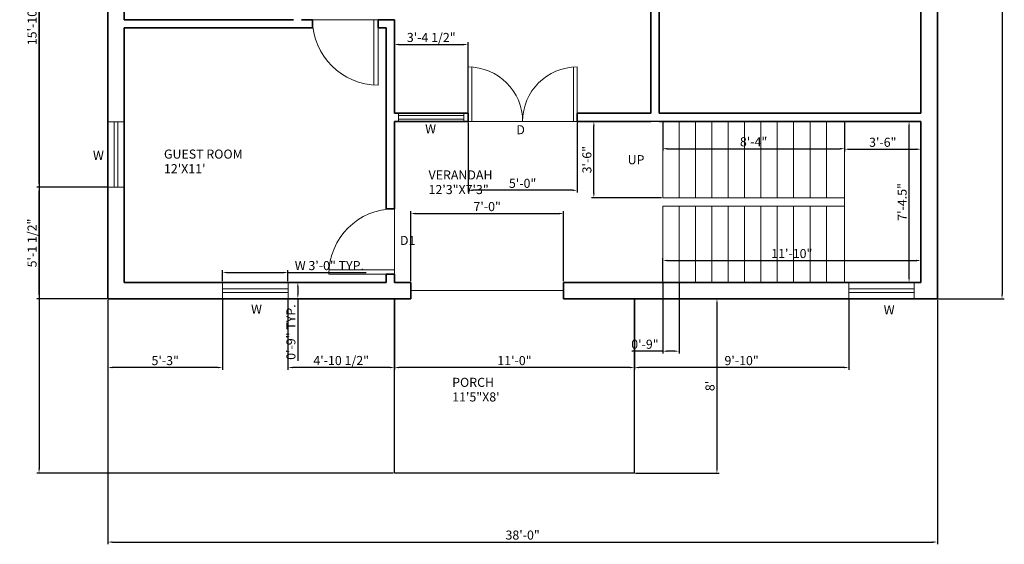
# Model space of a CAD drawing. Units: inches. Extents: x 2488 to 3029, y 1951 to 2721.
# Tile 1 of 2: x 2488 to 3029, y 1951 to 2239. Entities that reach past the tile are written whole.
import ezdxf

# ---------------------------------------------------------------- set-up
doc = ezdxf.new("R2010")
doc.units = ezdxf.units.IN
doc.header["$LTSCALE"] = 0.4
for name, color, linetype, lineweight in [('A-ANNO-DIMS', 52, 'Continuous', 18), ('A-ANNO-SYMB', 52, 'Continuous', 18), ('A-ANNO-TEXT', 52, 'Continuous', 18), ('A-AREA-IDEN', 52, 'Continuous', 18), ('A-FLOR-OTLN', 5, 'Continuous', 25), ('A-FLOR-STRS', 5, 'Continuous', 18), ('A-FLOR-THRS', 4, 'ZIGZAG', 18), ('A-GLAZ-JAMB', 8, 'ZIGZAG', 18), ('doors', 4, 'Continuous', 18), ('wall', 5, 'Continuous', 35), ('windows', 8, 'Continuous', 18)]:
    doc.layers.add(name, color=color, linetype=linetype, lineweight=lineweight)
doc.styles.get("Standard").update_dxf_attribs({"font": 'arial.ttf', "height": 5})
doc.linetypes.add('ZIGZAG', pattern='A,0.00254,-5.08,[131,ltypeshp.shx,S=5.08,R=0,X=-5.08,Y=0],-10.16,[131,ltypeshp.shx,S=5.08,R=180,X=5.08,Y=0],-5.08', length=20.32254)
doc.dimstyles.new('ISO-25', dxfattribs={"dimtxt": 5, "dimasz": 2.5, "dimexe": 1.25, "dimexo": 0.625, "dimtad": 1, "dimlunit": 3, "dimtxsty": 'Standard', "dimcen": 2.5, "dimadec": 0, "dimazin": 0, "dimtfac": 1, "dimtmove": 0, "dimatfit": 3, "dimfxl": 1, "dimarcsym": 0})

# ---------------------------------------------------------------- blocks, each defined once
blk = doc.blocks.new('*D1')
at = {"layer": 'A-ANNO-DIMS', "color": 0, "lineweight": -2, "transparency": 16777216}
for p, q in [((2841.37, 2182.57), (2841.37, 2166.96)), ((2941.37, 2182.57), (2941.37, 2166.96)), ((2843.87, 2168.21), (2938.87, 2168.21))]:
    blk.add_line(p, q, dxfattribs=at)
at = {"layer": 'A-ANNO-DIMS', "color": 0, "lineweight": 100, "transparency": 16777216}
for points in [[(2843.87, 2168.62), (2843.87, 2167.79), (2841.37, 2168.21)], [(2938.87, 2168.62), (2938.87, 2167.79), (2941.37, 2168.21)]]:
    blk.add_solid(points, dxfattribs=at)
at = {"layer": 'Defpoints', "color": 0, "lineweight": 100, "transparency": 16777216}
for p in [(2841.37, 2183.19), (2941.37, 2183.19), (2941.37, 2168.21)]:
    blk.add_point(p, dxfattribs=at)
at = {"layer": 'A-ANNO-DIMS', "color": 0, "transparency": 16777216, "insert": (2891.37, 2171.38), "char_height": 5, "attachment_point": 5}
blk.add_mtext('8\'-4"', dxfattribs=at)
blk = doc.blocks.new('*D2')
at = {"layer": 'A-ANNO-DIMS', "color": 0, "lineweight": -2, "transparency": 16777216}
for p, q in [((2941.37, 2182.57), (2941.37, 2166.68)), ((2983.37, 2182.57), (2983.37, 2166.68)), ((2943.87, 2167.93), (2980.87, 2167.93))]:
    blk.add_line(p, q, dxfattribs=at)
at = {"layer": 'A-ANNO-DIMS', "color": 0, "lineweight": 100, "transparency": 16777216}
for points in [[(2943.87, 2168.34), (2943.87, 2167.51), (2941.37, 2167.93)], [(2980.87, 2168.34), (2980.87, 2167.51), (2983.37, 2167.93)]]:
    blk.add_solid(points, dxfattribs=at)
at = {"layer": 'Defpoints', "color": 0, "lineweight": 100, "transparency": 16777216}
for p in [(2941.37, 2183.19), (2983.37, 2183.19), (2983.37, 2167.93)]:
    blk.add_point(p, dxfattribs=at)
at = {"layer": 'A-ANNO-DIMS', "color": 0, "transparency": 16777216, "insert": (2962.37, 2171.11), "char_height": 5, "attachment_point": 5}
blk.add_mtext('3\'-6"', dxfattribs=at)
blk = doc.blocks.new('*D3')
at = {"layer": 'A-ANNO-DIMS', "color": 0, "lineweight": -2, "transparency": 16777216}
for p, q in [((2982.75, 2183.19), (2975.57, 2183.19)), ((2976.82, 2097.19), (2976.82, 2180.69)), ((2982.75, 2094.69), (2975.57, 2094.69))]:
    blk.add_line(p, q, dxfattribs=at)
at = {"layer": 'A-ANNO-DIMS', "color": 0, "lineweight": 100, "transparency": 16777216}
for points in [[(2976.41, 2180.69), (2977.24, 2180.69), (2976.82, 2183.19)], [(2976.41, 2097.19), (2977.24, 2097.19), (2976.82, 2094.69)]]:
    blk.add_solid(points, dxfattribs=at)
at = {"layer": 'Defpoints', "color": 0, "lineweight": 100, "transparency": 16777216}
for p in [(2976.82, 2183.19), (2983.37, 2183.19), (2983.37, 2094.69)]:
    blk.add_point(p, dxfattribs=at)
at = {"layer": 'A-ANNO-DIMS', "color": 0, "transparency": 16777216, "insert": (2973.66, 2138.94), "char_height": 5, "attachment_point": 5, "rotation": 90}
blk.add_mtext('7\'-4.5"', dxfattribs=at)
blk = doc.blocks.new('*D4')
at = {"layer": 'A-ANNO-DIMS', "color": 0, "lineweight": -2, "transparency": 16777216}
for p, q in [((2841.37, 2095.32), (2841.37, 2107.97)), ((2843.87, 2106.72), (2980.87, 2106.72)), ((2983.37, 2095.32), (2983.37, 2107.97))]:
    blk.add_line(p, q, dxfattribs=at)
at = {"layer": 'A-ANNO-DIMS', "color": 0, "lineweight": 100, "transparency": 16777216}
for points in [[(2843.87, 2107.14), (2843.87, 2106.31), (2841.37, 2106.72)], [(2980.87, 2107.14), (2980.87, 2106.31), (2983.37, 2106.72)]]:
    blk.add_solid(points, dxfattribs=at)
at = {"layer": 'Defpoints', "color": 0, "lineweight": 100, "transparency": 16777216}
for p in [(2983.37, 2106.72), (2841.37, 2094.69), (2983.37, 2094.69)]:
    blk.add_point(p, dxfattribs=at)
at = {"layer": 'A-ANNO-DIMS', "color": 0, "transparency": 16777216, "insert": (2912.37, 2109.9), "char_height": 5, "attachment_point": 5}
blk.add_mtext('11\'-10"', dxfattribs=at)
blk = doc.blocks.new('*D5')
at = {"layer": 'A-ANNO-DIMS', "color": 0, "lineweight": -2, "transparency": 16777216}
for p, q in [((2826.5, 2085.69), (2872.45, 2085.69)), ((2871.2, 2083.19), (2871.2, 1992.19)), ((2826.5, 1989.69), (2872.45, 1989.69))]:
    blk.add_line(p, q, dxfattribs=at)
at = {"layer": 'A-ANNO-DIMS', "color": 0, "lineweight": 100, "transparency": 16777216}
for points in [[(2870.78, 2083.19), (2871.62, 2083.19), (2871.2, 2085.69)], [(2870.78, 1992.19), (2871.62, 1992.19), (2871.2, 1989.69)]]:
    blk.add_solid(points, dxfattribs=at)
at = {"layer": 'Defpoints', "color": 0, "lineweight": 100, "transparency": 16777216}
for p in [(2825.87, 2085.69), (2825.87, 1989.69), (2871.2, 1989.69)]:
    blk.add_point(p, dxfattribs=at)
at = {"layer": 'A-ANNO-DIMS', "color": 0, "transparency": 16777216, "insert": (2868.02, 2037.69), "char_height": 5, "attachment_point": 5, "rotation": 90}
blk.add_mtext("8'", dxfattribs=at)
blk = doc.blocks.new('*D6')
at = {"layer": 'A-ANNO-DIMS', "color": 0, "lineweight": -2, "transparency": 16777216}
for p, q in [((2993, 2625.69), (3029.19, 2625.69)), ((3027.94, 2623.19), (3027.94, 2088.19)), ((2993, 2085.69), (3029.19, 2085.69))]:
    blk.add_line(p, q, dxfattribs=at)
at = {"layer": 'A-ANNO-DIMS', "color": 0, "lineweight": 100, "transparency": 16777216}
for points in [[(3027.52, 2623.19), (3028.36, 2623.19), (3027.94, 2625.69)], [(3027.52, 2088.19), (3028.36, 2088.19), (3027.94, 2085.69)]]:
    blk.add_solid(points, dxfattribs=at)
at = {"layer": 'Defpoints', "color": 0, "lineweight": 100, "transparency": 16777216}
for p in [(2992.37, 2625.69), (2992.37, 2085.69), (3027.94, 2085.69)]:
    blk.add_point(p, dxfattribs=at)
at = {"layer": 'A-ANNO-DIMS', "color": 0, "transparency": 16777216, "insert": (3024.77, 2355.69), "char_height": 5, "attachment_point": 5, "rotation": 90}
blk.add_mtext("45'", dxfattribs=at)
blk = doc.blocks.new('WIN-36IN-9IN-WALL')
for p, q in [((0, 36), (0, 0)), ((9, 36), (0, 36)), ((3.5, 36), (3.5, 0)), ((5.5, 36), (5.5, 0)), ((9, 0), (9, 36)), ((0, 0), (9, 0))]:
    blk.add_line(p, q)
blk = doc.blocks.new('DOOR-SWING-30IN')
for p, q in [((28, 29.93), (28, 0)), ((30, 30), (30, 0)), ((30, 0), (0, 0))]:
    blk.add_line(p, q)
blk.add_arc((30, 0), 30, 90, 180)
blk = doc.blocks.new('DOOR-SWING-36IN')
for p, q in [((33.6, 35.92), (33.6, 0)), ((36, 36), (36, 0)), ((36, 0), (0, 0))]:
    blk.add_line(p, q)
blk.add_arc((36, 0), 36, 90, 180)
blk = doc.blocks.new('*D11')
at = {"layer": 'A-ANNO-DIMS', "color": 0, "lineweight": -2, "transparency": 16777216}
for p, q in [((2599.37, 2095.32), (2599.37, 2101.34)), ((2635.37, 2095.32), (2635.37, 2101.34)), ((2601.87, 2100.09), (2632.87, 2100.09)), ((2635.37, 2100.09), (2678.34, 2100.09))]:
    blk.add_line(p, q, dxfattribs=at)
at = {"layer": 'A-ANNO-DIMS', "color": 0, "lineweight": 100, "transparency": 16777216}
for points in [[(2601.87, 2100.51), (2601.87, 2099.68), (2599.37, 2100.09)], [(2632.87, 2100.51), (2632.87, 2099.68), (2635.37, 2100.09)]]:
    blk.add_solid(points, dxfattribs=at)
at = {"layer": 'Defpoints', "color": 0, "lineweight": 100, "transparency": 16777216}
for p in [(2635.37, 2100.09), (2599.37, 2094.69), (2635.37, 2094.69)]:
    blk.add_point(p, dxfattribs=at)
at = {"layer": 'A-ANNO-DIMS', "color": 0, "transparency": 16777216, "insert": (2658.11, 2103.27), "char_height": 5, "attachment_point": 5}
blk.add_mtext('W 3\'-0" TYP.', dxfattribs=at)
blk = doc.blocks.new('*D12')
at = {"layer": 'A-ANNO-DIMS', "color": 0, "lineweight": -2, "transparency": 16777216}
for p, q in [((2636, 2094.69), (2642.02, 2094.69)), ((2640.77, 2092.19), (2640.77, 2088.19)), ((2636, 2085.69), (2642.02, 2085.69)), ((2640.77, 2085.69), (2640.77, 2051.47))]:
    blk.add_line(p, q, dxfattribs=at)
at = {"layer": 'A-ANNO-DIMS', "color": 0, "lineweight": 100, "transparency": 16777216}
for points in [[(2640.36, 2092.19), (2641.19, 2092.19), (2640.77, 2094.69)], [(2640.36, 2088.19), (2641.19, 2088.19), (2640.77, 2085.69)]]:
    blk.add_solid(points, dxfattribs=at)
at = {"layer": 'Defpoints', "color": 0, "lineweight": 100, "transparency": 16777216}
for p in [(2635.37, 2094.69), (2635.37, 2085.69), (2640.77, 2085.69)]:
    blk.add_point(p, dxfattribs=at)
at = {"layer": 'A-ANNO-DIMS', "color": 0, "transparency": 16777216, "insert": (2637.6, 2067.33), "char_height": 5, "attachment_point": 5, "rotation": 90}
blk.add_mtext('0\'-9" TYP.', dxfattribs=at)
blk = doc.blocks.new('*D20')
at = {"layer": 'A-ANNO-DIMS', "color": 0, "lineweight": -2, "transparency": 16777216}
for p, q in [((2535.75, 2147.03), (2497.27, 2147.03)), ((2498.52, 2088.19), (2498.52, 2144.53)), ((2535.75, 2085.69), (2497.27, 2085.69))]:
    blk.add_line(p, q, dxfattribs=at)
at = {"layer": 'A-ANNO-DIMS', "color": 0, "lineweight": 100, "transparency": 16777216}
for points in [[(2498.11, 2144.53), (2498.94, 2144.53), (2498.52, 2147.03)], [(2498.11, 2088.19), (2498.94, 2088.19), (2498.52, 2085.69)]]:
    blk.add_solid(points, dxfattribs=at)
at = {"layer": 'Defpoints', "color": 0, "lineweight": 100, "transparency": 16777216}
for p in [(2498.52, 2147.03), (2536.37, 2147.03), (2536.37, 2085.69)]:
    blk.add_point(p, dxfattribs=at)
at = {"layer": 'A-ANNO-DIMS', "color": 0, "transparency": 16777216, "insert": (2495.31, 2116.36), "char_height": 5, "attachment_point": 5, "rotation": 90}
blk.add_mtext('5\'-1 1/2"', dxfattribs=at)
blk = doc.blocks.new('*D21')
at = {"layer": 'A-ANNO-DIMS', "color": 0, "lineweight": -2, "transparency": 16777216}
for p, q in [((2535.75, 2337.69), (2497.27, 2337.69)), ((2498.52, 2149.53), (2498.52, 2335.19)), ((2535.75, 2147.03), (2497.27, 2147.03))]:
    blk.add_line(p, q, dxfattribs=at)
at = {"layer": 'A-ANNO-DIMS', "color": 0, "lineweight": 100, "transparency": 16777216}
for points in [[(2498.11, 2335.19), (2498.94, 2335.19), (2498.52, 2337.69)], [(2498.11, 2149.53), (2498.94, 2149.53), (2498.52, 2147.03)]]:
    blk.add_solid(points, dxfattribs=at)
at = {"layer": 'Defpoints', "color": 0, "lineweight": 100, "transparency": 16777216}
for p in [(2498.52, 2337.69), (2536.37, 2337.69), (2536.37, 2147.03)]:
    blk.add_point(p, dxfattribs=at)
at = {"layer": 'A-ANNO-DIMS', "color": 0, "transparency": 16777216, "insert": (2495.31, 2242.36), "char_height": 5, "attachment_point": 5, "rotation": 90}
blk.add_mtext('15\'-10 1/2"', dxfattribs=at)
blk = doc.blocks.new('*D26')
at = {"layer": 'A-ANNO-DIMS', "color": 0, "lineweight": -2, "transparency": 16777216}
for p, q in [((2536.37, 2085.07), (2536.37, 2046.59)), ((2599.37, 2085.07), (2599.37, 2046.59)), ((2596.87, 2047.84), (2538.87, 2047.84))]:
    blk.add_line(p, q, dxfattribs=at)
at = {"layer": 'A-ANNO-DIMS', "color": 0, "lineweight": 100, "transparency": 16777216}
for points in [[(2538.87, 2048.26), (2538.87, 2047.43), (2536.37, 2047.84)], [(2596.87, 2048.26), (2596.87, 2047.43), (2599.37, 2047.84)]]:
    blk.add_solid(points, dxfattribs=at)
at = {"layer": 'Defpoints', "color": 0, "lineweight": 100, "transparency": 16777216}
for p in [(2536.37, 2085.69), (2599.37, 2085.69), (2536.37, 2047.84)]:
    blk.add_point(p, dxfattribs=at)
at = {"layer": 'A-ANNO-DIMS', "color": 0, "transparency": 16777216, "insert": (2567.87, 2051.02), "char_height": 5, "attachment_point": 5}
blk.add_mtext('5\'-3"', dxfattribs=at)
blk = doc.blocks.new('*D27')
at = {"layer": 'A-ANNO-DIMS', "color": 0, "lineweight": -2, "transparency": 16777216}
for p, q in [((2635.37, 2085.07), (2635.37, 2046.59)), ((2693.87, 2085.07), (2693.87, 2046.59)), ((2691.37, 2047.84), (2637.87, 2047.84))]:
    blk.add_line(p, q, dxfattribs=at)
at = {"layer": 'A-ANNO-DIMS', "color": 0, "lineweight": 100, "transparency": 16777216}
for points in [[(2637.87, 2048.26), (2637.87, 2047.43), (2635.37, 2047.84)], [(2691.37, 2048.26), (2691.37, 2047.43), (2693.87, 2047.84)]]:
    blk.add_solid(points, dxfattribs=at)
at = {"layer": 'Defpoints', "color": 0, "lineweight": 100, "transparency": 16777216}
for p in [(2635.37, 2085.69), (2693.87, 2085.69), (2635.37, 2047.84)]:
    blk.add_point(p, dxfattribs=at)
at = {"layer": 'A-ANNO-DIMS', "color": 0, "transparency": 16777216, "insert": (2664.62, 2051.05), "char_height": 5, "attachment_point": 5}
blk.add_mtext('4\'-10 1/2"', dxfattribs=at)
blk = doc.blocks.new('*D28')
at = {"layer": 'A-ANNO-DIMS', "color": 0, "lineweight": -2, "transparency": 16777216}
for p, q in [((2693.87, 2085.07), (2693.87, 2046.59)), ((2825.87, 2085.07), (2825.87, 2046.59)), ((2823.37, 2047.84), (2696.37, 2047.84))]:
    blk.add_line(p, q, dxfattribs=at)
at = {"layer": 'A-ANNO-DIMS', "color": 0, "lineweight": 100, "transparency": 16777216}
for points in [[(2696.37, 2048.26), (2696.37, 2047.43), (2693.87, 2047.84)], [(2823.37, 2048.26), (2823.37, 2047.43), (2825.87, 2047.84)]]:
    blk.add_solid(points, dxfattribs=at)
at = {"layer": 'Defpoints', "color": 0, "lineweight": 100, "transparency": 16777216}
for p in [(2693.87, 2085.69), (2825.87, 2085.69), (2693.87, 2047.84)]:
    blk.add_point(p, dxfattribs=at)
at = {"layer": 'A-ANNO-DIMS', "color": 0, "transparency": 16777216, "insert": (2759.87, 2051.02), "char_height": 5, "attachment_point": 5}
blk.add_mtext('11\'-0"', dxfattribs=at)
blk = doc.blocks.new('*D29')
at = {"layer": 'A-ANNO-DIMS', "color": 0, "lineweight": -2, "transparency": 16777216}
for p, q in [((2825.87, 2085.07), (2825.87, 2046.59)), ((2943.65, 2085.07), (2943.65, 2046.59)), ((2941.15, 2047.84), (2828.37, 2047.84))]:
    blk.add_line(p, q, dxfattribs=at)
at = {"layer": 'A-ANNO-DIMS', "color": 0, "lineweight": 100, "transparency": 16777216}
for points in [[(2828.37, 2048.26), (2828.37, 2047.43), (2825.87, 2047.84)], [(2941.15, 2048.26), (2941.15, 2047.43), (2943.65, 2047.84)]]:
    blk.add_solid(points, dxfattribs=at)
at = {"layer": 'Defpoints', "color": 0, "lineweight": 100, "transparency": 16777216}
for p in [(2825.87, 2085.69), (2943.65, 2085.69), (2825.87, 2047.84)]:
    blk.add_point(p, dxfattribs=at)
at = {"layer": 'A-ANNO-DIMS', "color": 0, "transparency": 16777216, "insert": (2884.76, 2051.02), "char_height": 5, "attachment_point": 5}
blk.add_mtext('9\'-10"', dxfattribs=at)
blk = doc.blocks.new('*D30')
at = {"layer": 'A-ANNO-DIMS', "color": 0, "lineweight": -2, "transparency": 16777216}
for p, q in [((2536.37, 2085.07), (2536.37, 1950.59)), ((2992.37, 2085.07), (2992.37, 1950.59)), ((2538.87, 1951.84), (2989.87, 1951.84))]:
    blk.add_line(p, q, dxfattribs=at)
at = {"layer": 'A-ANNO-DIMS', "color": 0, "lineweight": 100, "transparency": 16777216}
for points in [[(2538.87, 1952.26), (2538.87, 1951.43), (2536.37, 1951.84)], [(2989.87, 1952.26), (2989.87, 1951.43), (2992.37, 1951.84)]]:
    blk.add_solid(points, dxfattribs=at)
at = {"layer": 'Defpoints', "color": 0, "lineweight": 100, "transparency": 16777216}
for p in [(2536.37, 2085.69), (2992.37, 2085.69), (2992.37, 1951.84)]:
    blk.add_point(p, dxfattribs=at)
at = {"layer": 'A-ANNO-DIMS', "color": 0, "transparency": 16777216, "insert": (2764.37, 1955.02), "char_height": 5, "attachment_point": 5}
blk.add_mtext('38\'-0"', dxfattribs=at)
blk = doc.blocks.new('*D31')
at = {"layer": 'A-ANNO-DIMS', "color": 0, "lineweight": -2, "transparency": 16777216}
for p, q in [((2535.75, 2625.69), (2497.27, 2625.69)), ((2498.52, 2623.19), (2498.52, 1992.19)), ((2693.25, 1989.69), (2497.27, 1989.69))]:
    blk.add_line(p, q, dxfattribs=at)
at = {"layer": 'A-ANNO-DIMS', "color": 0, "lineweight": 100, "transparency": 16777216}
for points in [[(2498.11, 2623.19), (2498.94, 2623.19), (2498.52, 2625.69)], [(2498.11, 1992.19), (2498.94, 1992.19), (2498.52, 1989.69)]]:
    blk.add_solid(points, dxfattribs=at)
at = {"layer": 'Defpoints', "color": 0, "lineweight": 100, "transparency": 16777216}
for p in [(2536.37, 2625.69), (2498.52, 1989.69), (2693.87, 1989.69)]:
    blk.add_point(p, dxfattribs=at)
at = {"layer": 'A-ANNO-DIMS', "color": 0, "transparency": 16777216, "insert": (2495.34, 2307.69), "char_height": 5, "attachment_point": 5, "rotation": 90}
blk.add_mtext('53\'-0"', dxfattribs=at)
blk = doc.blocks.new('*D36')
at = {"layer": 'A-ANNO-DIMS', "color": 0, "lineweight": -2, "transparency": 16777216}
for p, q in [((2734.37, 2182.57), (2734.37, 2144.09)), ((2794.37, 2182.57), (2794.37, 2144.09)), ((2791.87, 2145.34), (2736.87, 2145.34))]:
    blk.add_line(p, q, dxfattribs=at)
at = {"layer": 'A-ANNO-DIMS', "color": 0, "lineweight": 100, "transparency": 16777216}
for points in [[(2736.87, 2145.76), (2736.87, 2144.93), (2734.37, 2145.34)], [(2791.87, 2145.76), (2791.87, 2144.93), (2794.37, 2145.34)]]:
    blk.add_solid(points, dxfattribs=at)
at = {"layer": 'Defpoints', "color": 0, "lineweight": 100, "transparency": 16777216}
for p in [(2734.37, 2183.19), (2794.37, 2183.19), (2734.37, 2145.34)]:
    blk.add_point(p, dxfattribs=at)
at = {"layer": 'A-ANNO-DIMS', "color": 0, "transparency": 16777216, "insert": (2764.37, 2148.52), "char_height": 5, "attachment_point": 5}
blk.add_mtext('5\'-0"', dxfattribs=at)
blk = doc.blocks.new('*D37')
at = {"layer": 'A-ANNO-DIMS', "color": 0, "lineweight": -2, "transparency": 16777216}
for p, q in [((2702.87, 2095.32), (2702.87, 2133.79)), ((2786.87, 2095.32), (2786.87, 2133.79)), ((2705.37, 2132.54), (2784.37, 2132.54))]:
    blk.add_line(p, q, dxfattribs=at)
at = {"layer": 'A-ANNO-DIMS', "color": 0, "lineweight": 100, "transparency": 16777216}
for points in [[(2705.37, 2132.96), (2705.37, 2132.13), (2702.87, 2132.54)], [(2784.37, 2132.96), (2784.37, 2132.13), (2786.87, 2132.54)]]:
    blk.add_solid(points, dxfattribs=at)
at = {"layer": 'Defpoints', "color": 0, "lineweight": 100, "transparency": 16777216}
for p in [(2786.87, 2132.54), (2702.87, 2094.69), (2786.87, 2094.69)]:
    blk.add_point(p, dxfattribs=at)
at = {"layer": 'A-ANNO-DIMS', "color": 0, "transparency": 16777216, "insert": (2744.87, 2135.72), "char_height": 5, "attachment_point": 5}
blk.add_mtext('7\'-0"', dxfattribs=at)
blk = doc.blocks.new('*D38')
at = {"layer": 'A-ANNO-DIMS', "color": 0, "lineweight": -2, "transparency": 16777216}
for p, q in [((2693.87, 2188.32), (2693.87, 2226.79)), ((2696.37, 2225.54), (2731.87, 2225.54)), ((2734.37, 2188.32), (2734.37, 2226.79))]:
    blk.add_line(p, q, dxfattribs=at)
at = {"layer": 'A-ANNO-DIMS', "color": 0, "lineweight": 100, "transparency": 16777216}
for points in [[(2696.37, 2225.96), (2696.37, 2225.13), (2693.87, 2225.54)], [(2731.87, 2225.96), (2731.87, 2225.13), (2734.37, 2225.54)]]:
    blk.add_solid(points, dxfattribs=at)
at = {"layer": 'Defpoints', "color": 0, "lineweight": 100, "transparency": 16777216}
for p in [(2734.37, 2225.54), (2693.87, 2187.69), (2734.37, 2187.69)]:
    blk.add_point(p, dxfattribs=at)
at = {"layer": 'A-ANNO-DIMS', "color": 0, "transparency": 16777216, "insert": (2714.12, 2228.76), "char_height": 5, "attachment_point": 5}
blk.add_mtext('3\'-4 1/2"', dxfattribs=at)
blk = doc.blocks.new('*D39')
at = {"layer": 'A-ANNO-DIMS', "color": 0, "lineweight": -2, "transparency": 16777216}
for p, q in [((2841.37, 2094.07), (2841.37, 2055.59)), ((2850.37, 2094.07), (2850.37, 2055.59)), ((2841.37, 2056.84), (2824.33, 2056.84)), ((2847.87, 2056.84), (2843.87, 2056.84))]:
    blk.add_line(p, q, dxfattribs=at)
at = {"layer": 'A-ANNO-DIMS', "color": 0, "lineweight": 100, "transparency": 16777216}
for points in [[(2843.87, 2057.26), (2843.87, 2056.43), (2841.37, 2056.84)], [(2847.87, 2057.26), (2847.87, 2056.43), (2850.37, 2056.84)]]:
    blk.add_solid(points, dxfattribs=at)
at = {"layer": 'Defpoints', "color": 0, "lineweight": 100, "transparency": 16777216}
for p in [(2841.37, 2094.69), (2850.37, 2094.69), (2841.37, 2056.84)]:
    blk.add_point(p, dxfattribs=at)
at = {"layer": 'A-ANNO-DIMS', "color": 0, "transparency": 16777216, "insert": (2831.6, 2060.02), "char_height": 5, "attachment_point": 5}
blk.add_mtext('0\'-9"', dxfattribs=at)
blk = doc.blocks.new('*D40')
at = {"layer": 'A-ANNO-DIMS', "color": 0, "lineweight": -2, "transparency": 16777216}
for p, q in [((2840.75, 2183.19), (2802.27, 2183.19)), ((2803.52, 2143.69), (2803.52, 2180.69)), ((2840.75, 2141.19), (2802.27, 2141.19))]:
    blk.add_line(p, q, dxfattribs=at)
at = {"layer": 'A-ANNO-DIMS', "color": 0, "lineweight": 100, "transparency": 16777216}
for points in [[(2803.11, 2180.69), (2803.94, 2180.69), (2803.52, 2183.19)], [(2803.11, 2143.69), (2803.94, 2143.69), (2803.52, 2141.19)]]:
    blk.add_solid(points, dxfattribs=at)
at = {"layer": 'Defpoints', "color": 0, "lineweight": 100, "transparency": 16777216}
for p in [(2803.52, 2183.19), (2841.37, 2183.19), (2841.37, 2141.19)]:
    blk.add_point(p, dxfattribs=at)
at = {"layer": 'A-ANNO-DIMS', "color": 0, "transparency": 16777216, "insert": (2800.34, 2162.19), "char_height": 5, "attachment_point": 5, "rotation": 90}
blk.add_mtext('3\'-6"', dxfattribs=at)

msp = doc.modelspace()

# ---------------------------------------------------------------- linework, layer by layer
at = {"layer": 'A-ANNO-SYMB'}
msp.add_lwpolyline([(2831.723, 2161.799, 0, 0, 0), (2855.877, 2161.799, 10, 0, 0), (2864.435, 2161.799, 0, 0, 0)], format="xyseb", dxfattribs=at)
at = {"layer": 'A-FLOR-OTLN'}
for p, q in [((2693.874, 1989.694), (2693.874, 2085.694)), ((2825.874, 1989.694), (2825.874, 2085.694)), ((2825.874, 1989.694), (2693.874, 1989.694))]:
    msp.add_line(p, q, dxfattribs=at)
at = {"layer": 'A-FLOR-STRS'}
for p, q in [((2841.374, 2183.194), (2841.374, 2141.194)), ((2850.374, 2183.194), (2850.374, 2141.194)), ((2859.374, 2183.194), (2859.374, 2141.194)), ((2868.374, 2183.194), (2868.374, 2141.194)), ((2877.374, 2183.194), (2877.374, 2141.194)), ((2886.374, 2183.194), (2886.374, 2141.194)), ((2895.374, 2183.194), (2895.374, 2141.194)), ((2904.374, 2183.194), (2904.374, 2141.194)), ((2913.374, 2183.194), (2913.374, 2141.194)), ((2922.374, 2183.194), (2922.374, 2141.194)), ((2931.374, 2183.194), (2931.374, 2141.194)), ((2941.374, 2183.194), (2941.374, 2094.694)), ((2841.374, 2141.194), (2941.374, 2141.194)), ((2941.374, 2136.694), (2841.374, 2136.694)), ((2841.374, 2136.694), (2841.374, 2094.694)), ((2850.374, 2136.694), (2850.374, 2094.694)), ((2859.374, 2136.694), (2859.374, 2094.694)), ((2868.374, 2136.694), (2868.374, 2094.694)), ((2877.374, 2136.694), (2877.374, 2094.694)), ((2886.374, 2136.694), (2886.374, 2094.694)), ((2895.374, 2136.694), (2895.374, 2094.694)), ((2904.374, 2136.694), (2904.374, 2094.694)), ((2913.374, 2136.694), (2913.374, 2094.694)), ((2922.374, 2136.694), (2922.374, 2094.694)), ((2931.374, 2136.694), (2931.374, 2094.694))]:
    msp.add_line(p, q, dxfattribs=at)
at = {"layer": 'A-FLOR-THRS'}
msp.add_line((2702.874, 2090.194), (2786.874, 2090.194), dxfattribs=at)
at = {"layer": 'A-GLAZ-JAMB'}
for p, q in [((2696.124, 2187.694), (2696.124, 2183.194)), ((2732.124, 2187.694), (2732.124, 2183.194))]:
    msp.add_line(p, q, dxfattribs=at)
at = {"layer": 'wall'}
for p, q in [((2536.374, 2085.694), (2536.374, 2625.694)), ((2992.374, 2625.694), (2992.374, 2085.694)), ((2834.874, 2187.694), (2834.874, 2331.694)), ((2839.374, 2187.694), (2839.374, 2331.694)), ((2983.374, 2331.694), (2983.374, 2187.694)), ((2545.374, 2239.194), (2545.374, 2287.194)), ((2545.374, 2239.194), (2638.374, 2239.194)), ((2642.874, 2239.194), (2648.874, 2239.194)), ((2648.874, 2234.694), (2648.874, 2239.194)), ((2684.874, 2234.694), (2684.874, 2239.194)), ((2684.874, 2239.194), (2693.874, 2239.194)), ((2693.874, 2187.694), (2693.874, 2239.194)), ((2545.374, 2094.694), (2545.374, 2234.694)), ((2545.374, 2234.694), (2648.874, 2234.694)), ((2684.874, 2234.694), (2689.374, 2234.694)), ((2689.374, 2135.194), (2689.374, 2234.694)), ((2693.874, 2187.694), (2734.374, 2187.694)), ((2734.374, 2187.694), (2734.374, 2183.194)), ((2794.374, 2187.694), (2794.374, 2183.194)), ((2794.374, 2187.694), (2834.874, 2187.694)), ((2839.374, 2187.694), (2983.374, 2187.694)), ((2693.874, 2183.194), (2734.374, 2183.194)), ((2693.874, 2135.194), (2693.874, 2183.194)), ((2794.374, 2183.194), (2834.874, 2183.194)), ((2839.374, 2183.194), (2983.374, 2183.194)), ((2983.374, 2183.194), (2983.374, 2094.694)), ((2689.374, 2135.194), (2693.874, 2135.194)), ((2689.374, 2094.694), (2689.374, 2099.194)), ((2689.374, 2099.194), (2693.874, 2099.194)), ((2693.874, 2094.694), (2693.874, 2099.194)), ((2689.374, 2094.694), (2545.374, 2094.694)), ((2702.874, 2094.694), (2693.874, 2094.694)), ((2702.874, 2094.694), (2702.874, 2085.694)), ((2983.374, 2094.694), (2786.874, 2094.694)), ((2786.874, 2094.694), (2786.874, 2085.694)), ((2702.874, 2085.694), (2536.374, 2085.694)), ((2992.374, 2085.694), (2786.874, 2085.694))]:
    msp.add_line(p, q, dxfattribs=at)
at = {"layer": 'windows'}
for p, q in [((2696.124, 2187.694), (2732.124, 2187.694)), ((2696.124, 2186.444), (2732.124, 2186.444)), ((2696.124, 2184.444), (2732.124, 2184.444)), ((2696.124, 2183.194), (2732.124, 2183.194))]:
    msp.add_line(p, q, dxfattribs=at)

# ---------------------------------------------------------------- block references
at = {"layer": 'doors', "extrusion": (0, 0, -1), "zscale": -1}
for p, rotation in [((-2648.874, 2239.194), 180), ((-2693.874, 2135.194), 270.0000000000063)]:
    msp.add_blockref('DOOR-SWING-36IN', p, dxfattribs=dict(at, rotation=rotation))
msp.add_blockref('DOOR-SWING-30IN', (-2764.374, 2183.194), dxfattribs=at)
at = {"layer": 'doors'}
msp.add_blockref('DOOR-SWING-30IN', (2764.374, 2183.194), dxfattribs=at)
at = {"layer": 'windows'}
for p, rotation in [((2545.374, 2183.028), 180), ((2599.374, 2094.694), 270.0000000000045), ((2943.646, 2094.694), 270.0000000000007)]:
    msp.add_blockref('WIN-36IN-9IN-WALL', p, dxfattribs=dict(at, rotation=rotation))

# ---------------------------------------------------------------- texts
at = {"layer": 'A-ANNO-TEXT'}
for s, p in [('W', (2710.788, 2176.643)), ('D', (2760.9, 2176.16)), ('W', (2528.144, 2162.05)), ('UP', (2822.106, 2159.679)), ('D1', (2696.922, 2115.275)), ('W', (2615.063, 2077.448)), ('W', (2962.873, 2077.053))]:
    msp.add_text(s, height=5, dxfattribs=at).set_placement(p)
at = {"layer": 'A-AREA-IDEN'}
for s, p in [('GUEST ROOM', (2567.169, 2162.756)), ("12'X11'", (2567.169, 2154.724)), ('VERANDAH', (2712.651, 2151.284)), ('12\'3"X7\'3"', (2712.651, 2143.252)), ('PORCH', (2725.635, 2037.193)), ('11\'5"X8\'', (2725.635, 2029.161))]:
    msp.add_text(s, height=5, dxfattribs=at).set_placement(p)

# ---------------------------------------------------------------- dimensions: what is measured, and where the dimension line sits
at = {"layer": 'A-ANNO-DIMS'}
for base, p1, p2, angle, override, picture, middle in [((2498.524, 1989.694), (2536.374, 2625.694), (2693.874, 1989.694), 90, {"dimdec": 1, "dimlfac": 1, "dimrnd": 0, "dimzin": 1, "dimdsep": 46, "dimlunit": 4, "dimfrac": 2}, '*D31', (2495.344, 2307.694)), ((3027.941, 2085.694), (2992.374, 2625.694), (2992.374, 2085.694), 90, {"dimclrd": 0, "dimclre": 0, "dimclrt": 0}, '*D6', (3024.773, 2355.694)), ((2498.524, 2337.694), (2536.374, 2147.028), (2536.374, 2337.694), 90, {"dimdec": 1, "dimlfac": 1, "dimrnd": 0, "dimzin": 1, "dimdsep": 46, "dimlunit": 4, "dimfrac": 2}, '*D21', (2495.313, 2242.361)), ((2734.374, 2145.344), (2794.374, 2183.194), (2734.374, 2183.194), 180, {"dimdec": 1, "dimlfac": 1, "dimrnd": 0, "dimzin": 1, "dimdsep": 46, "dimlunit": 4, "dimfrac": 2}, '*D36', (2764.374, 2148.522)), ((2803.524, 2183.194), (2841.374, 2141.194), (2841.374, 2183.194), 90, {"dimdec": 1, "dimlfac": 1, "dimrnd": 0, "dimzin": 1, "dimdsep": 46, "dimlunit": 4, "dimfrac": 2}, '*D40', (2800.344, 2162.194)), ((2976.823, 2183.194), (2983.374, 2094.694), (2983.374, 2183.194), 90, {"dimclrd": 0, "dimclre": 0, "dimclrt": 0}, '*D3', (2973.655, 2138.944)), ((2498.524, 2147.028), (2536.374, 2085.694), (2536.374, 2147.028), 90, {"dimdec": 1, "dimlfac": 1, "dimrnd": 0, "dimzin": 1, "dimdsep": 46, "dimlunit": 4, "dimfrac": 2}, '*D20', (2495.313, 2116.361)), ((2841.374, 2056.844), (2850.374, 2094.694), (2841.374, 2094.694), 180, {"dimdec": 1, "dimlfac": 1, "dimrnd": 0, "dimzin": 1, "dimdsep": 46, "dimlunit": 4, "dimfrac": 2}, '*D39', (2831.603, 2060.022)), ((2536.374, 2047.844), (2599.374, 2085.694), (2536.374, 2085.694), 180, {"dimdec": 1, "dimlfac": 1, "dimrnd": 0, "dimzin": 1, "dimdsep": 46, "dimlunit": 4, "dimfrac": 2}, '*D26', (2567.874, 2051.023)), ((2635.374, 2047.844), (2693.874, 2085.694), (2635.374, 2085.694), 180, {"dimdec": 1, "dimlfac": 1, "dimrnd": 0, "dimzin": 1, "dimdsep": 46, "dimlunit": 4, "dimfrac": 2}, '*D27', (2664.624, 2051.054)), ((2693.874, 2047.844), (2825.874, 2085.694), (2693.874, 2085.694), 180, {"dimdec": 1, "dimlfac": 1, "dimrnd": 0, "dimzin": 1, "dimdsep": 46, "dimlunit": 4, "dimfrac": 2}, '*D28', (2759.874, 2051.022)), ((2871.201, 1989.694), (2825.874, 2085.694), (2825.874, 1989.694), 90, {"dimclrd": 0, "dimclre": 0, "dimclrt": 0}, '*D5', (2868.023, 2037.694)), ((2825.874, 2047.844), (2943.646, 2085.694), (2825.874, 2085.694), 180, {"dimdec": 1, "dimlfac": 1, "dimrnd": 0, "dimzin": 1, "dimdsep": 46, "dimlunit": 4, "dimfrac": 2}, '*D29', (2884.76, 2051.022))]:
    dim = msp.add_linear_dim(base=base, p1=p1, p2=p2, angle=angle, dimstyle='ISO-25', override=override, dxfattribs=at)
    dim.commit()
    dim.dimension.update_dxf_attribs({"geometry": picture, "text_midpoint": middle})
for base, p1, p2, override, picture, middle in [((2734.374, 2225.544), (2693.874, 2187.694), (2734.374, 2187.694), {"dimdec": 1, "dimlfac": 1, "dimrnd": 0, "dimzin": 1, "dimdsep": 46, "dimlunit": 4, "dimfrac": 2}, '*D38', (2714.124, 2228.756)), ((2941.374, 2168.205), (2841.374, 2183.194), (2941.374, 2183.194), {"dimclrd": 0, "dimclre": 0, "dimclrt": 0}, '*D1', (2891.374, 2171.383)), ((2983.374, 2167.927), (2941.374, 2183.194), (2983.374, 2183.194), {"dimclrd": 0, "dimclre": 0, "dimclrt": 0}, '*D2', (2962.374, 2171.107)), ((2786.874, 2132.544), (2702.874, 2094.694), (2786.874, 2094.694), {"dimdec": 1, "dimlfac": 1, "dimrnd": 0, "dimzin": 1, "dimdsep": 46, "dimlunit": 4, "dimfrac": 2}, '*D37', (2744.874, 2135.722)), ((2983.374, 2106.725), (2841.374, 2094.694), (2983.374, 2094.694), {"dimclrd": 0, "dimclre": 0, "dimclrt": 0}, '*D4', (2912.374, 2109.903)), ((2992.374, 1951.844), (2536.374, 2085.694), (2992.374, 2085.694), {"dimdec": 1, "dimlfac": 1, "dimrnd": 0, "dimzin": 1, "dimdsep": 46, "dimlunit": 4, "dimfrac": 2}, '*D30', (2764.374, 1955.023))]:
    dim = msp.add_linear_dim(base=base, p1=p1, p2=p2, dimstyle='ISO-25', override=override, dxfattribs=at)
    dim.commit()
    dim.dimension.update_dxf_attribs({"geometry": picture, "text_midpoint": middle})
for base, p1, p2, angle, text, picture, middle in [((2635.374, 2100.094), (2599.374, 2094.694), (2635.374, 2094.694), 0, 'W <> TYP.', '*D11', (2658.106, 2103.273)), ((2640.774, 2085.694), (2635.374, 2094.694), (2635.374, 2085.694), 270, '<> TYP.', '*D12', (2637.596, 2067.33))]:
    dim = msp.add_linear_dim(base=base, p1=p1, p2=p2, angle=angle, text=text, dimstyle='ISO-25', override={"dimdec": 1, "dimlfac": 1, "dimrnd": 0, "dimzin": 1, "dimdsep": 46, "dimlunit": 4, "dimfrac": 2}, dxfattribs=at)
    dim.commit()
    dim.dimension.update_dxf_attribs({"geometry": picture, "text_midpoint": middle})

doc.saveas('drawing.dxf')
